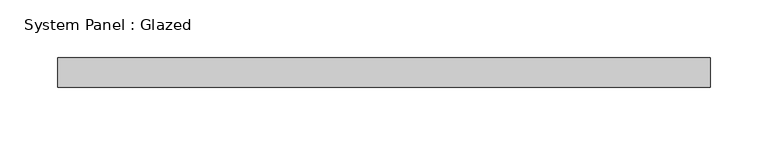
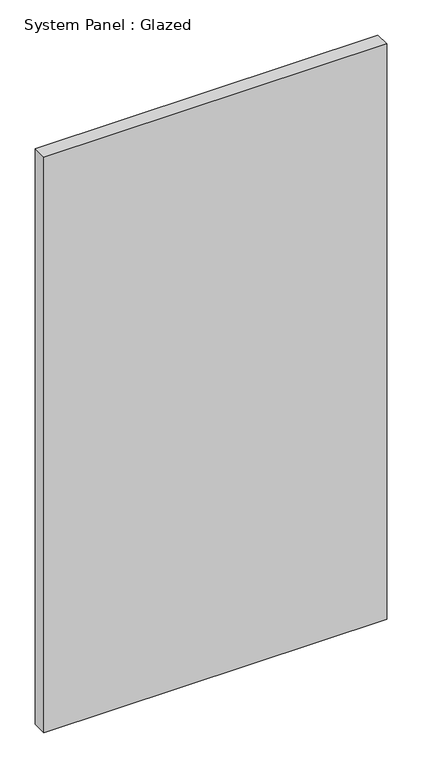
"""IFC4 building model written with IfcOpenShell, lengths in millimetres: plate geometry, System Panel : Glazed."""

from ifc_helpers import new_model, si_unit, origin, origin_with_axes, place, context, project, spatial, polyline, outline, extrude, source, transform, mapped, element, save


def system_panel_glazed_fbef02e7(model_context):
    return source(origin(), model_context, "Body", "SweptSolid", [
        extrude(outline(polyline([(282.575, -44.45), (-282.575, -44.45), (-282.575, -19.05), (282.575, -19.05), (282.575, -44.45)])), origin_with_axes(), (0.0, 0.0, 1.0), 1003.3),
    ])


if __name__ == "__main__":
    model = new_model("IFC4")
    model_context = context("Model", 3, world=origin())
    ifc_project = project(units=[si_unit("LENGTHUNIT", "METRE", prefix="MILLI")], contexts=[model_context])
    site = spatial("IfcSite", under=ifc_project)
    building = spatial("IfcBuilding", under=site)
    placement = place(None, origin())
    system_panel_glazed_shape = system_panel_glazed_fbef02e7(model_context)
    element("IfcPlate", 1, ObjectType="System Panel : Glazed", at=placement, inside=building, context=model_context, shape_type="MappedRepresentation", body=[
        mapped(system_panel_glazed_shape, transform((0.0, 0.0, 0.0), x_axis=(1.0, 0.0, 0.0), y_axis=(0.0, 1.0, 0.0), z_axis=(0.0, 0.0, 1.0))),
    ])
    save(model, "model.ifc")

# Revit data of these elements
# Type "System Panel : Glazed"
#   Construction Type Id = "GSP4R"
#   Analytic Construction = "1/8 in Pilkington single glazing"
#   Visual Light Transmittance = 0.9
#   Solar Heat Gain Coefficient = 0.86
#   Heat Transfer Coefficient (U) = 1.18115 BTU/(h·ft²·°F)
#   Define Thermal Properties by = 1
# Element 1 (IfcPlate, "System Panel : Glazed")
#   Materials on its faces: "Glass"
# Materials
#   "Glass": class "Glass", colour RGB 0 128 192, transparency 0.75, Description = "Soda Lime Glass", Cost = 0
